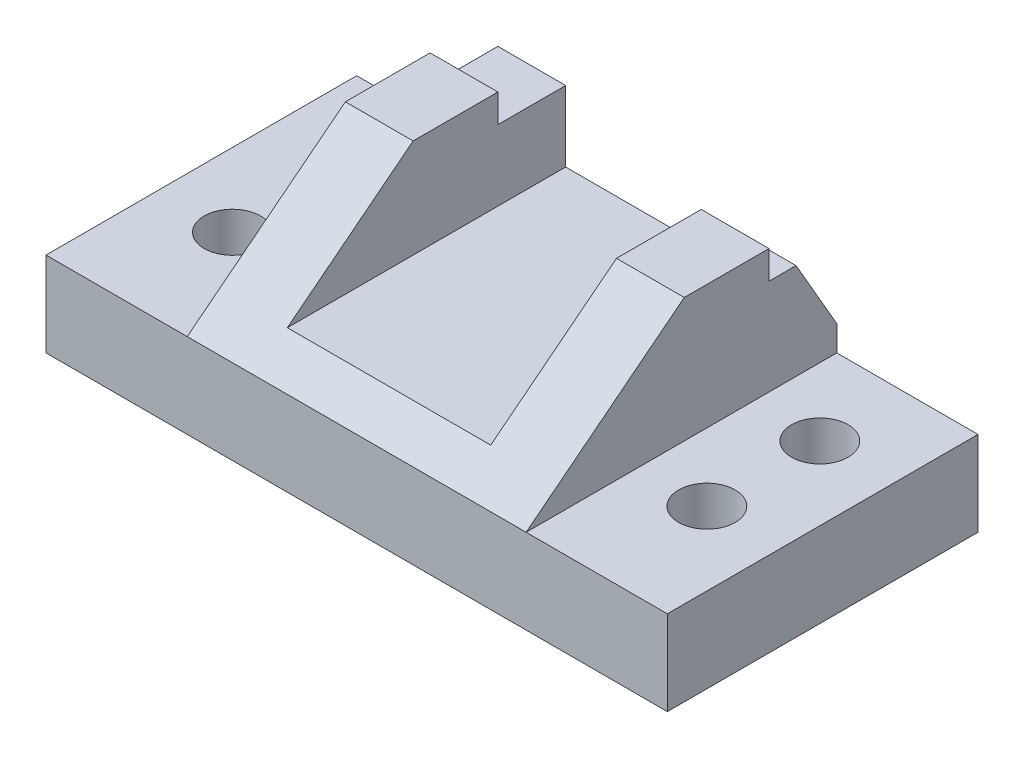
ISO-10303-21;
HEADER;
FILE_DESCRIPTION(('STEP AP214'),'2;1');
FILE_NAME('part.step','',(''),(''),'','','');
FILE_SCHEMA(('AUTOMOTIVE_DESIGN { 1 0 10303 214 1 1 1 1 }'));
ENDSEC;
DATA;
#1=APPLICATION_CONTEXT('core data for automotive mechanical design processes');
#2=APPLICATION_PROTOCOL_DEFINITION('international standard','automotive_design',2000,#1);
#3=PRODUCT_CONTEXT('',#1,'mechanical');
#4=PRODUCT('Part','Part','',(#3));
#5=PRODUCT_RELATED_PRODUCT_CATEGORY('part','',(#4));
#6=PRODUCT_DEFINITION_FORMATION('','',#4);
#7=PRODUCT_DEFINITION_CONTEXT('part definition',#1,'design');
#8=PRODUCT_DEFINITION('design','',#6,#7);
#9=PRODUCT_DEFINITION_SHAPE('','',#8);
#10=(LENGTH_UNIT() NAMED_UNIT(*) SI_UNIT(.MILLI.,.METRE.));
#11=(NAMED_UNIT(*) PLANE_ANGLE_UNIT() SI_UNIT($,.RADIAN.));
#12=(NAMED_UNIT(*) SI_UNIT($,.STERADIAN.) SOLID_ANGLE_UNIT());
#13=UNCERTAINTY_MEASURE_WITH_UNIT(LENGTH_MEASURE(1.E-05),#10,'distance_accuracy_value','');
#14=(GEOMETRIC_REPRESENTATION_CONTEXT(3) GLOBAL_UNCERTAINTY_ASSIGNED_CONTEXT((#13)) GLOBAL_UNIT_ASSIGNED_CONTEXT((#10,
#11,#12)) REPRESENTATION_CONTEXT('',''));
#15=CARTESIAN_POINT('',(0.,0.,0.));
#16=DIRECTION('',(0.,0.,1.));
#17=DIRECTION('',(1.,0.,0.));
#18=AXIS2_PLACEMENT_3D('',#15,#16,#17);
#19=CARTESIAN_POINT('',(0.,15.,0.));
#20=DIRECTION('',(0.,-1.,0.));
#21=DIRECTION('',(0.,0.,-1.));
#22=AXIS2_PLACEMENT_3D('',#19,#20,#21);
#23=PLANE('',#22);
#24=CARTESIAN_POINT('',(42.,15.,-40.));
#25=DIRECTION('',(0.,1.,0.));
#26=DIRECTION('',(0.,0.,-1.));
#27=AXIS2_PLACEMENT_3D('',#24,#25,#26);
#28=CIRCLE('',#27,5.);
#29=CARTESIAN_POINT('',(42.,15.,-45.));
#30=VERTEX_POINT('',#29);
#31=EDGE_CURVE('E229',#30,#30,#28,.T.);
#32=ORIENTED_EDGE('',*,*,#31,.F.);
#33=EDGE_LOOP('',(#32));
#34=FACE_BOUND('',#33,.T.);
#35=CARTESIAN_POINT('',(42.,15.,-20.));
#36=DIRECTION('',(0.,1.,0.));
#37=DIRECTION('',(0.,0.,-1.));
#38=AXIS2_PLACEMENT_3D('',#35,#36,#37);
#39=CIRCLE('',#38,5.);
#40=CARTESIAN_POINT('',(42.,15.,-25.));
#41=VERTEX_POINT('',#40);
#42=EDGE_CURVE('E231',#41,#41,#39,.T.);
#43=ORIENTED_EDGE('',*,*,#42,.F.);
#44=EDGE_LOOP('',(#43));
#45=FACE_BOUND('',#44,.T.);
#46=DIRECTION('',(0.,0.,-1.));
#47=VECTOR('',#46,1.);
#48=CARTESIAN_POINT('',(30.,15.,63.9061812346818));
#49=LINE('',#48,#47);
#50=CARTESIAN_POINT('',(30.,15.,0.));
#51=VERTEX_POINT('',#50);
#52=CARTESIAN_POINT('',(30.,15.,-55.));
#53=VERTEX_POINT('',#52);
#54=EDGE_CURVE('E202',#51,#53,#49,.T.);
#55=ORIENTED_EDGE('',*,*,#54,.F.);
#56=DIRECTION('',(1.,0.,0.));
#57=VECTOR('',#56,1.);
#58=CARTESIAN_POINT('',(-55.,15.,0.));
#59=LINE('',#58,#57);
#60=CARTESIAN_POINT('',(55.,15.,0.));
#61=VERTEX_POINT('',#60);
#62=EDGE_CURVE('E254',#51,#61,#59,.T.);
#63=ORIENTED_EDGE('',*,*,#62,.T.);
#64=DIRECTION('',(0.,0.,-1.));
#65=VECTOR('',#64,1.);
#66=CARTESIAN_POINT('',(55.,15.,0.));
#67=LINE('',#66,#65);
#68=CARTESIAN_POINT('',(55.,15.,-55.));
#69=VERTEX_POINT('',#68);
#70=EDGE_CURVE('E257',#61,#69,#67,.T.);
#71=ORIENTED_EDGE('',*,*,#70,.T.);
#72=DIRECTION('',(-1.,0.,0.));
#73=VECTOR('',#72,1.);
#74=CARTESIAN_POINT('',(-55.,15.,-55.));
#75=LINE('',#74,#73);
#76=EDGE_CURVE('E263',#69,#53,#75,.T.);
#77=ORIENTED_EDGE('',*,*,#76,.T.);
#78=EDGE_LOOP('',(#55,#63,#71,#77));
#79=FACE_BOUND('',#78,.T.);
#80=ADVANCED_FACE('F39',(#34,#45,#79),#23,.F.);
#81=CARTESIAN_POINT('',(-55.,15.,0.));
#82=VERTEX_POINT('',#81);
#83=CARTESIAN_POINT('',(-30.,15.,0.));
#84=VERTEX_POINT('',#83);
#85=EDGE_CURVE('E260',#82,#84,#59,.T.);
#86=ORIENTED_EDGE('',*,*,#85,.T.);
#87=DIRECTION('',(0.,0.,-1.));
#88=VECTOR('',#87,1.);
#89=CARTESIAN_POINT('',(-30.,15.,63.9061812346818));
#90=LINE('',#89,#88);
#91=CARTESIAN_POINT('',(-30.,15.,-55.));
#92=VERTEX_POINT('',#91);
#93=EDGE_CURVE('E223',#84,#92,#90,.T.);
#94=ORIENTED_EDGE('',*,*,#93,.T.);
#95=CARTESIAN_POINT('',(-55.,15.,-55.));
#96=VERTEX_POINT('',#95);
#97=EDGE_CURVE('E265',#92,#96,#75,.T.);
#98=ORIENTED_EDGE('',*,*,#97,.T.);
#99=DIRECTION('',(0.,0.,1.));
#100=VECTOR('',#99,1.);
#101=CARTESIAN_POINT('',(-55.,15.,0.));
#102=LINE('',#101,#100);
#103=EDGE_CURVE('E252',#96,#82,#102,.T.);
#104=ORIENTED_EDGE('',*,*,#103,.T.);
#105=EDGE_LOOP('',(#86,#94,#98,#104));
#106=FACE_BOUND('',#105,.T.);
#107=CARTESIAN_POINT('',(-42.,15.,-40.));
#108=DIRECTION('',(0.,1.,0.));
#109=DIRECTION('',(0.,0.,1.));
#110=AXIS2_PLACEMENT_3D('',#107,#108,#109);
#111=CIRCLE('',#110,5.);
#112=CARTESIAN_POINT('',(-42.,15.,-35.));
#113=VERTEX_POINT('',#112);
#114=EDGE_CURVE('E247',#113,#113,#111,.T.);
#115=ORIENTED_EDGE('',*,*,#114,.F.);
#116=EDGE_LOOP('',(#115));
#117=FACE_BOUND('',#116,.T.);
#118=CARTESIAN_POINT('',(-42.,15.,-20.));
#119=DIRECTION('',(0.,1.,0.));
#120=DIRECTION('',(0.,0.,1.));
#121=AXIS2_PLACEMENT_3D('',#118,#119,#120);
#122=CIRCLE('',#121,5.);
#123=CARTESIAN_POINT('',(-42.,15.,-15.));
#124=VERTEX_POINT('',#123);
#125=EDGE_CURVE('E238',#124,#124,#122,.T.);
#126=ORIENTED_EDGE('',*,*,#125,.F.);
#127=EDGE_LOOP('',(#126));
#128=FACE_BOUND('',#127,.T.);
#129=ADVANCED_FACE('F302',(#106,#117,#128),#23,.F.);
#130=CARTESIAN_POINT('',(0.,0.,0.));
#131=DIRECTION('',(0.,-1.,0.));
#132=DIRECTION('',(0.,0.,-1.));
#133=AXIS2_PLACEMENT_3D('',#130,#131,#132);
#134=PLANE('',#133);
#135=CARTESIAN_POINT('',(42.,0.,-20.));
#136=DIRECTION('',(0.,1.,0.));
#137=DIRECTION('',(0.,0.,-1.));
#138=AXIS2_PLACEMENT_3D('',#135,#136,#137);
#139=CIRCLE('',#138,5.);
#140=CARTESIAN_POINT('',(42.,0.,-25.));
#141=VERTEX_POINT('',#140);
#142=EDGE_CURVE('E232',#141,#141,#139,.T.);
#143=ORIENTED_EDGE('',*,*,#142,.T.);
#144=EDGE_LOOP('',(#143));
#145=FACE_BOUND('',#144,.T.);
#146=CARTESIAN_POINT('',(-42.,0.,-40.));
#147=DIRECTION('',(0.,1.,0.));
#148=DIRECTION('',(0.,0.,1.));
#149=AXIS2_PLACEMENT_3D('',#146,#147,#148);
#150=CIRCLE('',#149,5.);
#151=CARTESIAN_POINT('',(-42.,0.,-35.));
#152=VERTEX_POINT('',#151);
#153=EDGE_CURVE('E244',#152,#152,#150,.T.);
#154=ORIENTED_EDGE('',*,*,#153,.T.);
#155=EDGE_LOOP('',(#154));
#156=FACE_BOUND('',#155,.T.);
#157=DIRECTION('',(0.,0.,1.));
#158=VECTOR('',#157,1.);
#159=CARTESIAN_POINT('',(-55.,0.,0.));
#160=LINE('',#159,#158);
#161=CARTESIAN_POINT('',(-55.,0.,-55.));
#162=VERTEX_POINT('',#161);
#163=CARTESIAN_POINT('',(-55.,0.,0.));
#164=VERTEX_POINT('',#163);
#165=EDGE_CURVE('E246',#162,#164,#160,.T.);
#166=ORIENTED_EDGE('',*,*,#165,.F.);
#167=DIRECTION('',(-1.,0.,0.));
#168=VECTOR('',#167,1.);
#169=CARTESIAN_POINT('',(-55.,0.,-55.));
#170=LINE('',#169,#168);
#171=CARTESIAN_POINT('',(55.,0.,-55.));
#172=VERTEX_POINT('',#171);
#173=EDGE_CURVE('E258',#172,#162,#170,.T.);
#174=ORIENTED_EDGE('',*,*,#173,.F.);
#175=DIRECTION('',(0.,0.,-1.));
#176=VECTOR('',#175,1.);
#177=CARTESIAN_POINT('',(55.,0.,0.));
#178=LINE('',#177,#176);
#179=CARTESIAN_POINT('',(55.,0.,0.));
#180=VERTEX_POINT('',#179);
#181=EDGE_CURVE('E271',#180,#172,#178,.T.);
#182=ORIENTED_EDGE('',*,*,#181,.F.);
#183=DIRECTION('',(1.,0.,0.));
#184=VECTOR('',#183,1.);
#185=CARTESIAN_POINT('',(-55.,0.,0.));
#186=LINE('',#185,#184);
#187=EDGE_CURVE('E267',#164,#180,#186,.T.);
#188=ORIENTED_EDGE('',*,*,#187,.F.);
#189=EDGE_LOOP('',(#166,#174,#182,#188));
#190=FACE_BOUND('',#189,.T.);
#191=CARTESIAN_POINT('',(-42.,0.,-20.));
#192=DIRECTION('',(0.,1.,0.));
#193=DIRECTION('',(0.,0.,1.));
#194=AXIS2_PLACEMENT_3D('',#191,#192,#193);
#195=CIRCLE('',#194,5.);
#196=CARTESIAN_POINT('',(-42.,0.,-15.));
#197=VERTEX_POINT('',#196);
#198=EDGE_CURVE('E240',#197,#197,#195,.T.);
#199=ORIENTED_EDGE('',*,*,#198,.T.);
#200=EDGE_LOOP('',(#199));
#201=FACE_BOUND('',#200,.T.);
#202=CARTESIAN_POINT('',(42.,0.,-40.));
#203=DIRECTION('',(0.,1.,0.));
#204=DIRECTION('',(0.,0.,-1.));
#205=AXIS2_PLACEMENT_3D('',#202,#203,#204);
#206=CIRCLE('',#205,5.);
#207=CARTESIAN_POINT('',(42.,0.,-45.));
#208=VERTEX_POINT('',#207);
#209=EDGE_CURVE('E207',#208,#208,#206,.T.);
#210=ORIENTED_EDGE('',*,*,#209,.T.);
#211=EDGE_LOOP('',(#210));
#212=FACE_BOUND('',#211,.T.);
#213=ADVANCED_FACE('F288',(#145,#156,#190,#201,#212),#134,.T.);
#214=CARTESIAN_POINT('',(-55.,15.,0.));
#215=DIRECTION('',(1.,0.,0.));
#216=DIRECTION('',(0.,0.,-1.));
#217=AXIS2_PLACEMENT_3D('',#214,#215,#216);
#218=PLANE('',#217);
#219=ORIENTED_EDGE('',*,*,#165,.T.);
#220=DIRECTION('',(0.,-1.,0.));
#221=VECTOR('',#220,1.);
#222=CARTESIAN_POINT('',(-55.,15.,0.));
#223=LINE('',#222,#221);
#224=EDGE_CURVE('E11',#82,#164,#223,.T.);
#225=ORIENTED_EDGE('',*,*,#224,.F.);
#226=ORIENTED_EDGE('',*,*,#103,.F.);
#227=DIRECTION('',(0.,-1.,0.));
#228=VECTOR('',#227,1.);
#229=CARTESIAN_POINT('',(-55.,15.,-55.));
#230=LINE('',#229,#228);
#231=EDGE_CURVE('E266',#96,#162,#230,.T.);
#232=ORIENTED_EDGE('',*,*,#231,.T.);
#233=EDGE_LOOP('',(#219,#225,#226,#232));
#234=FACE_BOUND('',#233,.T.);
#235=ADVANCED_FACE('F41',(#234),#218,.F.);
#236=CARTESIAN_POINT('',(-55.,15.,0.));
#237=DIRECTION('',(0.,0.,-1.));
#238=DIRECTION('',(-1.,0.,0.));
#239=AXIS2_PLACEMENT_3D('',#236,#237,#238);
#240=PLANE('',#239);
#241=ORIENTED_EDGE('',*,*,#62,.F.);
#242=DIRECTION('',(-1.,0.,0.));
#243=VECTOR('',#242,1.);
#244=CARTESIAN_POINT('',(55.,15.,0.));
#245=LINE('',#244,#243);
#246=EDGE_CURVE('E318',#51,#84,#245,.T.);
#247=ORIENTED_EDGE('',*,*,#246,.T.);
#248=ORIENTED_EDGE('',*,*,#85,.F.);
#249=ORIENTED_EDGE('',*,*,#224,.T.);
#250=ORIENTED_EDGE('',*,*,#187,.T.);
#251=DIRECTION('',(0.,-1.,0.));
#252=VECTOR('',#251,1.);
#253=CARTESIAN_POINT('',(55.,15.,0.));
#254=LINE('',#253,#252);
#255=EDGE_CURVE('E50',#61,#180,#254,.T.);
#256=ORIENTED_EDGE('',*,*,#255,.F.);
#257=EDGE_LOOP('',(#241,#247,#248,#249,#250,#256));
#258=FACE_BOUND('',#257,.T.);
#259=ADVANCED_FACE('F358',(#258),#240,.F.);
#260=CARTESIAN_POINT('',(55.,15.,0.));
#261=DIRECTION('',(-1.,0.,0.));
#262=DIRECTION('',(0.,0.,1.));
#263=AXIS2_PLACEMENT_3D('',#260,#261,#262);
#264=PLANE('',#263);
#265=ORIENTED_EDGE('',*,*,#181,.T.);
#266=DIRECTION('',(0.,-1.,0.));
#267=VECTOR('',#266,1.);
#268=CARTESIAN_POINT('',(55.,15.,-55.));
#269=LINE('',#268,#267);
#270=EDGE_CURVE('E277',#69,#172,#269,.T.);
#271=ORIENTED_EDGE('',*,*,#270,.F.);
#272=ORIENTED_EDGE('',*,*,#70,.F.);
#273=ORIENTED_EDGE('',*,*,#255,.T.);
#274=EDGE_LOOP('',(#265,#271,#272,#273));
#275=FACE_BOUND('',#274,.T.);
#276=ADVANCED_FACE('F284',(#275),#264,.F.);
#277=CARTESIAN_POINT('',(-55.,15.,-55.));
#278=DIRECTION('',(0.,0.,1.));
#279=DIRECTION('',(1.,0.,0.));
#280=AXIS2_PLACEMENT_3D('',#277,#278,#279);
#281=PLANE('',#280);
#282=DIRECTION('',(1.,0.,0.));
#283=VECTOR('',#282,1.);
#284=CARTESIAN_POINT('',(-18.,19.5,-55.));
#285=LINE('',#284,#283);
#286=CARTESIAN_POINT('',(-18.,19.5,-55.));
#287=VERTEX_POINT('',#286);
#288=CARTESIAN_POINT('',(18.,19.5,-55.));
#289=VERTEX_POINT('',#288);
#290=EDGE_CURVE('E205',#287,#289,#285,.T.);
#291=ORIENTED_EDGE('',*,*,#290,.T.);
#292=DIRECTION('',(-1.,0.,0.));
#293=VECTOR('',#292,1.);
#294=CARTESIAN_POINT('',(44.4337567297406,19.5,-55.));
#295=LINE('',#294,#293);
#296=CARTESIAN_POINT('',(30.,19.5,-55.));
#297=VERTEX_POINT('',#296);
#298=EDGE_CURVE('E161',#297,#289,#295,.T.);
#299=ORIENTED_EDGE('',*,*,#298,.F.);
#300=DIRECTION('',(0.,-1.,0.));
#301=VECTOR('',#300,1.);
#302=CARTESIAN_POINT('',(30.,15.,-55.));
#303=LINE('',#302,#301);
#304=EDGE_CURVE('E168',#297,#53,#303,.T.);
#305=ORIENTED_EDGE('',*,*,#304,.T.);
#306=ORIENTED_EDGE('',*,*,#76,.F.);
#307=ORIENTED_EDGE('',*,*,#270,.T.);
#308=ORIENTED_EDGE('',*,*,#173,.T.);
#309=ORIENTED_EDGE('',*,*,#231,.F.);
#310=ORIENTED_EDGE('',*,*,#97,.F.);
#311=DIRECTION('',(0.,1.,0.));
#312=VECTOR('',#311,1.);
#313=CARTESIAN_POINT('',(-30.,15.,-55.));
#314=LINE('',#313,#312);
#315=CARTESIAN_POINT('',(-30.,32.,-55.));
#316=VERTEX_POINT('',#315);
#317=EDGE_CURVE('E197',#92,#316,#314,.T.);
#318=ORIENTED_EDGE('',*,*,#317,.T.);
#319=DIRECTION('',(-1.,0.,0.));
#320=VECTOR('',#319,1.);
#321=CARTESIAN_POINT('',(55.,32.,-55.));
#322=LINE('',#321,#320);
#323=CARTESIAN_POINT('',(-18.,32.,-55.));
#324=VERTEX_POINT('',#323);
#325=EDGE_CURVE('E62',#324,#316,#322,.T.);
#326=ORIENTED_EDGE('',*,*,#325,.F.);
#327=DIRECTION('',(0.,-1.,0.));
#328=VECTOR('',#327,1.);
#329=CARTESIAN_POINT('',(-18.,19.5,-55.));
#330=LINE('',#329,#328);
#331=EDGE_CURVE('E199',#324,#287,#330,.T.);
#332=ORIENTED_EDGE('',*,*,#331,.T.);
#333=EDGE_LOOP('',(#291,#299,#305,#306,#307,#308,#309,#310,#318,#326,#332));
#334=FACE_BOUND('',#333,.T.);
#335=ADVANCED_FACE('F294',(#334),#281,.F.);
#336=CARTESIAN_POINT('',(-42.,15.,-40.));
#337=DIRECTION('',(0.,-1.,0.));
#338=DIRECTION('',(0.,0.,-1.));
#339=AXIS2_PLACEMENT_3D('',#336,#337,#338);
#340=CYLINDRICAL_SURFACE('',#339,5.);
#341=ORIENTED_EDGE('',*,*,#114,.T.);
#342=EDGE_LOOP('',(#341));
#343=FACE_BOUND('',#342,.T.);
#344=ORIENTED_EDGE('',*,*,#153,.F.);
#345=EDGE_LOOP('',(#344));
#346=FACE_BOUND('',#345,.T.);
#347=ADVANCED_FACE('F377',(#343,#346),#340,.F.);
#348=CARTESIAN_POINT('',(-42.,15.,-20.));
#349=DIRECTION('',(0.,-1.,0.));
#350=DIRECTION('',(0.,0.,-1.));
#351=AXIS2_PLACEMENT_3D('',#348,#349,#350);
#352=CYLINDRICAL_SURFACE('',#351,5.);
#353=ORIENTED_EDGE('',*,*,#125,.T.);
#354=EDGE_LOOP('',(#353));
#355=FACE_BOUND('',#354,.T.);
#356=ORIENTED_EDGE('',*,*,#198,.F.);
#357=EDGE_LOOP('',(#356));
#358=FACE_BOUND('',#357,.T.);
#359=ADVANCED_FACE('F388',(#355,#358),#352,.F.);
#360=CARTESIAN_POINT('',(42.,15.,-20.));
#361=DIRECTION('',(0.,-1.,0.));
#362=DIRECTION('',(0.,0.,-1.));
#363=AXIS2_PLACEMENT_3D('',#360,#361,#362);
#364=CYLINDRICAL_SURFACE('',#363,5.);
#365=ORIENTED_EDGE('',*,*,#42,.T.);
#366=EDGE_LOOP('',(#365));
#367=FACE_BOUND('',#366,.T.);
#368=ORIENTED_EDGE('',*,*,#142,.F.);
#369=EDGE_LOOP('',(#368));
#370=FACE_BOUND('',#369,.T.);
#371=ADVANCED_FACE('F395',(#367,#370),#364,.F.);
#372=CARTESIAN_POINT('',(42.,15.,-40.));
#373=DIRECTION('',(0.,-1.,0.));
#374=DIRECTION('',(0.,0.,-1.));
#375=AXIS2_PLACEMENT_3D('',#372,#373,#374);
#376=CYLINDRICAL_SURFACE('',#375,5.);
#377=ORIENTED_EDGE('',*,*,#31,.T.);
#378=EDGE_LOOP('',(#377));
#379=FACE_BOUND('',#378,.T.);
#380=ORIENTED_EDGE('',*,*,#209,.F.);
#381=EDGE_LOOP('',(#380));
#382=FACE_BOUND('',#381,.T.);
#383=ADVANCED_FACE('F409',(#379,#382),#376,.F.);
#384=CARTESIAN_POINT('',(30.,15.,63.9061812346818));
#385=DIRECTION('',(1.,0.,0.));
#386=DIRECTION('',(0.,0.,-1.));
#387=AXIS2_PLACEMENT_3D('',#384,#385,#386);
#388=PLANE('',#387);
#389=DIRECTION('',(0.,0.866025403784442,0.499999999999995));
#390=VECTOR('',#389,1.);
#391=CARTESIAN_POINT('',(30.,19.5,-55.));
#392=LINE('',#391,#390);
#393=CARTESIAN_POINT('',(30.,32.,-47.7831216351298));
#394=VERTEX_POINT('',#393);
#395=EDGE_CURVE('E156',#297,#394,#392,.T.);
#396=ORIENTED_EDGE('',*,*,#395,.T.);
#397=DIRECTION('',(0.,0.,-1.));
#398=VECTOR('',#397,1.);
#399=CARTESIAN_POINT('',(30.,32.,63.9061812346818));
#400=LINE('',#399,#398);
#401=CARTESIAN_POINT('',(30.,32.,-43.));
#402=VERTEX_POINT('',#401);
#403=EDGE_CURVE('E169',#402,#394,#400,.T.);
#404=ORIENTED_EDGE('',*,*,#403,.F.);
#405=DIRECTION('',(0.,-1.,0.));
#406=VECTOR('',#405,1.);
#407=CARTESIAN_POINT('',(30.,15.,-43.));
#408=LINE('',#407,#406);
#409=CARTESIAN_POINT('',(30.,37.,-43.));
#410=VERTEX_POINT('',#409);
#411=EDGE_CURVE('E186',#410,#402,#408,.T.);
#412=ORIENTED_EDGE('',*,*,#411,.F.);
#413=DIRECTION('',(0.,0.,-1.));
#414=VECTOR('',#413,1.);
#415=CARTESIAN_POINT('',(30.,37.,63.9061812346818));
#416=LINE('',#415,#414);
#417=CARTESIAN_POINT('',(30.,37.,-28.));
#418=VERTEX_POINT('',#417);
#419=EDGE_CURVE('E206',#418,#410,#416,.T.);
#420=ORIENTED_EDGE('',*,*,#419,.F.);
#421=DIRECTION('',(0.,0.617821551931904,-0.786318338822423));
#422=VECTOR('',#421,1.);
#423=CARTESIAN_POINT('',(30.,-16.0459050793092,39.5129701009389));
#424=LINE('',#423,#422);
#425=EDGE_CURVE('E191',#51,#418,#424,.T.);
#426=ORIENTED_EDGE('',*,*,#425,.F.);
#427=ORIENTED_EDGE('',*,*,#54,.T.);
#428=ORIENTED_EDGE('',*,*,#304,.F.);
#429=EDGE_LOOP('',(#396,#404,#412,#420,#426,#427,#428));
#430=FACE_BOUND('',#429,.T.);
#431=ADVANCED_FACE('F167',(#430),#388,.T.);
#432=CARTESIAN_POINT('',(30.,37.,63.9061812346818));
#433=DIRECTION('',(0.,1.,0.));
#434=DIRECTION('',(0.,0.,1.));
#435=AXIS2_PLACEMENT_3D('',#432,#433,#434);
#436=PLANE('',#435);
#437=DIRECTION('',(-1.,0.,0.));
#438=VECTOR('',#437,1.);
#439=CARTESIAN_POINT('',(55.,37.,-28.));
#440=LINE('',#439,#438);
#441=CARTESIAN_POINT('',(18.,37.,-28.));
#442=VERTEX_POINT('',#441);
#443=EDGE_CURVE('E321',#418,#442,#440,.T.);
#444=ORIENTED_EDGE('',*,*,#443,.F.);
#445=ORIENTED_EDGE('',*,*,#419,.T.);
#446=DIRECTION('',(-1.,0.,0.));
#447=VECTOR('',#446,1.);
#448=CARTESIAN_POINT('',(55.,37.,-43.));
#449=LINE('',#448,#447);
#450=CARTESIAN_POINT('',(18.,37.,-43.));
#451=VERTEX_POINT('',#450);
#452=EDGE_CURVE('E327',#410,#451,#449,.T.);
#453=ORIENTED_EDGE('',*,*,#452,.T.);
#454=DIRECTION('',(0.,0.,-1.));
#455=VECTOR('',#454,1.);
#456=CARTESIAN_POINT('',(18.,37.,63.9061812346818));
#457=LINE('',#456,#455);
#458=EDGE_CURVE('E209',#442,#451,#457,.T.);
#459=ORIENTED_EDGE('',*,*,#458,.F.);
#460=EDGE_LOOP('',(#444,#445,#453,#459));
#461=FACE_BOUND('',#460,.T.);
#462=ADVANCED_FACE('F411',(#461),#436,.T.);
#463=CARTESIAN_POINT('',(18.,19.5,63.9061812346818));
#464=DIRECTION('',(-1.,0.,0.));
#465=DIRECTION('',(0.,0.,1.));
#466=AXIS2_PLACEMENT_3D('',#463,#464,#465);
#467=PLANE('',#466);
#468=DIRECTION('',(0.,0.866025403784442,0.499999999999995));
#469=VECTOR('',#468,1.);
#470=CARTESIAN_POINT('',(18.,19.5,-55.));
#471=LINE('',#470,#469);
#472=CARTESIAN_POINT('',(18.,32.,-47.7831216351298));
#473=VERTEX_POINT('',#472);
#474=EDGE_CURVE('E53',#289,#473,#471,.T.);
#475=ORIENTED_EDGE('',*,*,#474,.F.);
#476=DIRECTION('',(0.,0.,-1.));
#477=VECTOR('',#476,1.);
#478=CARTESIAN_POINT('',(18.,19.5,63.9061812346818));
#479=LINE('',#478,#477);
#480=CARTESIAN_POINT('',(18.,19.5,-5.72727272727275));
#481=VERTEX_POINT('',#480);
#482=EDGE_CURVE('E213',#481,#289,#479,.T.);
#483=ORIENTED_EDGE('',*,*,#482,.F.);
#484=DIRECTION('',(0.,-0.617821551931904,0.786318338822423));
#485=VECTOR('',#484,1.);
#486=CARTESIAN_POINT('',(18.,-14.3282394641672,37.3268502271219));
#487=LINE('',#486,#485);
#488=EDGE_CURVE('E194',#442,#481,#487,.T.);
#489=ORIENTED_EDGE('',*,*,#488,.F.);
#490=ORIENTED_EDGE('',*,*,#458,.T.);
#491=DIRECTION('',(0.,1.,0.));
#492=VECTOR('',#491,1.);
#493=CARTESIAN_POINT('',(18.,19.5,-43.));
#494=LINE('',#493,#492);
#495=CARTESIAN_POINT('',(18.,32.,-43.));
#496=VERTEX_POINT('',#495);
#497=EDGE_CURVE('E176',#496,#451,#494,.T.);
#498=ORIENTED_EDGE('',*,*,#497,.F.);
#499=DIRECTION('',(0.,0.,1.));
#500=VECTOR('',#499,1.);
#501=CARTESIAN_POINT('',(18.,32.,63.9061812346818));
#502=LINE('',#501,#500);
#503=EDGE_CURVE('E179',#473,#496,#502,.T.);
#504=ORIENTED_EDGE('',*,*,#503,.F.);
#505=EDGE_LOOP('',(#475,#483,#489,#490,#498,#504));
#506=FACE_BOUND('',#505,.T.);
#507=ADVANCED_FACE('F337',(#506),#467,.T.);
#508=CARTESIAN_POINT('',(-18.,19.5,63.9061812346818));
#509=DIRECTION('',(0.,1.,0.));
#510=DIRECTION('',(0.,0.,1.));
#511=AXIS2_PLACEMENT_3D('',#508,#509,#510);
#512=PLANE('',#511);
#513=DIRECTION('',(-1.,0.,0.));
#514=VECTOR('',#513,1.);
#515=CARTESIAN_POINT('',(-18.,19.5,-5.72727272727275));
#516=LINE('',#515,#514);
#517=CARTESIAN_POINT('',(-18.,19.5,-5.72727272727277));
#518=VERTEX_POINT('',#517);
#519=EDGE_CURVE('E190',#481,#518,#516,.T.);
#520=ORIENTED_EDGE('',*,*,#519,.F.);
#521=ORIENTED_EDGE('',*,*,#482,.T.);
#522=ORIENTED_EDGE('',*,*,#290,.F.);
#523=DIRECTION('',(0.,0.,-1.));
#524=VECTOR('',#523,1.);
#525=CARTESIAN_POINT('',(-18.,19.5,63.9061812346818));
#526=LINE('',#525,#524);
#527=EDGE_CURVE('E216',#518,#287,#526,.T.);
#528=ORIENTED_EDGE('',*,*,#527,.F.);
#529=EDGE_LOOP('',(#520,#521,#522,#528));
#530=FACE_BOUND('',#529,.T.);
#531=ADVANCED_FACE('F345',(#530),#512,.T.);
#532=CARTESIAN_POINT('',(-18.,19.5,63.9061812346818));
#533=DIRECTION('',(1.,0.,0.));
#534=DIRECTION('',(0.,1.,0.));
#535=AXIS2_PLACEMENT_3D('',#532,#533,#534);
#536=PLANE('',#535);
#537=DIRECTION('',(0.,0.617821551931904,-0.786318338822423));
#538=VECTOR('',#537,1.);
#539=CARTESIAN_POINT('',(-18.,-14.3282394641672,37.3268502271219));
#540=LINE('',#539,#538);
#541=CARTESIAN_POINT('',(-18.,37.,-28.));
#542=VERTEX_POINT('',#541);
#543=EDGE_CURVE('E189',#518,#542,#540,.T.);
#544=ORIENTED_EDGE('',*,*,#543,.F.);
#545=ORIENTED_EDGE('',*,*,#527,.T.);
#546=ORIENTED_EDGE('',*,*,#331,.F.);
#547=DIRECTION('',(0.,0.,-1.));
#548=VECTOR('',#547,1.);
#549=CARTESIAN_POINT('',(-18.,32.,63.9061812346818));
#550=LINE('',#549,#548);
#551=CARTESIAN_POINT('',(-18.,32.,-43.));
#552=VERTEX_POINT('',#551);
#553=EDGE_CURVE('E182',#552,#324,#550,.T.);
#554=ORIENTED_EDGE('',*,*,#553,.F.);
#555=DIRECTION('',(0.,-1.,0.));
#556=VECTOR('',#555,1.);
#557=CARTESIAN_POINT('',(-18.,19.5,-43.));
#558=LINE('',#557,#556);
#559=CARTESIAN_POINT('',(-18.,37.,-43.));
#560=VERTEX_POINT('',#559);
#561=EDGE_CURVE('E177',#560,#552,#558,.T.);
#562=ORIENTED_EDGE('',*,*,#561,.F.);
#563=DIRECTION('',(0.,0.,-1.));
#564=VECTOR('',#563,1.);
#565=CARTESIAN_POINT('',(-18.,37.,63.9061812346818));
#566=LINE('',#565,#564);
#567=EDGE_CURVE('E218',#542,#560,#566,.T.);
#568=ORIENTED_EDGE('',*,*,#567,.F.);
#569=EDGE_LOOP('',(#544,#545,#546,#554,#562,#568));
#570=FACE_BOUND('',#569,.T.);
#571=ADVANCED_FACE('F346',(#570),#536,.T.);
#572=CARTESIAN_POINT('',(-18.,37.,63.9061812346818));
#573=DIRECTION('',(0.,1.,0.));
#574=DIRECTION('',(-1.,0.,0.));
#575=AXIS2_PLACEMENT_3D('',#572,#573,#574);
#576=PLANE('',#575);
#577=CARTESIAN_POINT('',(-30.,37.,-28.));
#578=VERTEX_POINT('',#577);
#579=EDGE_CURVE('E314',#542,#578,#440,.T.);
#580=ORIENTED_EDGE('',*,*,#579,.F.);
#581=ORIENTED_EDGE('',*,*,#567,.T.);
#582=CARTESIAN_POINT('',(-30.,37.,-43.));
#583=VERTEX_POINT('',#582);
#584=EDGE_CURVE('E328',#560,#583,#449,.T.);
#585=ORIENTED_EDGE('',*,*,#584,.T.);
#586=DIRECTION('',(0.,0.,-1.));
#587=VECTOR('',#586,1.);
#588=CARTESIAN_POINT('',(-30.,37.,63.9061812346818));
#589=LINE('',#588,#587);
#590=EDGE_CURVE('E225',#578,#583,#589,.T.);
#591=ORIENTED_EDGE('',*,*,#590,.F.);
#592=EDGE_LOOP('',(#580,#581,#585,#591));
#593=FACE_BOUND('',#592,.T.);
#594=ADVANCED_FACE('F353',(#593),#576,.T.);
#595=CARTESIAN_POINT('',(-30.,15.,63.9061812346818));
#596=DIRECTION('',(-1.,0.,0.));
#597=DIRECTION('',(0.,0.,1.));
#598=AXIS2_PLACEMENT_3D('',#595,#596,#597);
#599=PLANE('',#598);
#600=DIRECTION('',(0.,-0.617821551931904,0.786318338822423));
#601=VECTOR('',#600,1.);
#602=CARTESIAN_POINT('',(-30.,15.,0.));
#603=LINE('',#602,#601);
#604=EDGE_CURVE('E315',#578,#84,#603,.T.);
#605=ORIENTED_EDGE('',*,*,#604,.F.);
#606=ORIENTED_EDGE('',*,*,#590,.T.);
#607=DIRECTION('',(0.,1.,0.));
#608=VECTOR('',#607,1.);
#609=CARTESIAN_POINT('',(-30.,37.,-43.));
#610=LINE('',#609,#608);
#611=CARTESIAN_POINT('',(-30.,32.,-43.));
#612=VERTEX_POINT('',#611);
#613=EDGE_CURVE('E309',#612,#583,#610,.T.);
#614=ORIENTED_EDGE('',*,*,#613,.F.);
#615=DIRECTION('',(0.,0.,1.));
#616=VECTOR('',#615,1.);
#617=CARTESIAN_POINT('',(-30.,32.,-43.));
#618=LINE('',#617,#616);
#619=EDGE_CURVE('E310',#316,#612,#618,.T.);
#620=ORIENTED_EDGE('',*,*,#619,.F.);
#621=ORIENTED_EDGE('',*,*,#317,.F.);
#622=ORIENTED_EDGE('',*,*,#93,.F.);
#623=EDGE_LOOP('',(#605,#606,#614,#620,#621,#622));
#624=FACE_BOUND('',#623,.T.);
#625=ADVANCED_FACE('F307',(#624),#599,.T.);
#626=CARTESIAN_POINT('',(55.,32.,-43.));
#627=DIRECTION('',(0.,-1.,0.));
#628=DIRECTION('',(0.,0.,-1.));
#629=AXIS2_PLACEMENT_3D('',#626,#627,#628);
#630=PLANE('',#629);
#631=ORIENTED_EDGE('',*,*,#553,.T.);
#632=ORIENTED_EDGE('',*,*,#325,.T.);
#633=ORIENTED_EDGE('',*,*,#619,.T.);
#634=DIRECTION('',(-1.,0.,0.));
#635=VECTOR('',#634,1.);
#636=CARTESIAN_POINT('',(55.,32.,-43.));
#637=LINE('',#636,#635);
#638=EDGE_CURVE('E330',#552,#612,#637,.T.);
#639=ORIENTED_EDGE('',*,*,#638,.F.);
#640=EDGE_LOOP('',(#631,#632,#633,#639));
#641=FACE_BOUND('',#640,.T.);
#642=ADVANCED_FACE('F423',(#641),#630,.F.);
#643=CARTESIAN_POINT('',(55.,37.,-43.));
#644=DIRECTION('',(0.,0.,1.));
#645=DIRECTION('',(1.,0.,0.));
#646=AXIS2_PLACEMENT_3D('',#643,#644,#645);
#647=PLANE('',#646);
#648=ORIENTED_EDGE('',*,*,#561,.T.);
#649=ORIENTED_EDGE('',*,*,#638,.T.);
#650=ORIENTED_EDGE('',*,*,#613,.T.);
#651=ORIENTED_EDGE('',*,*,#584,.F.);
#652=EDGE_LOOP('',(#648,#649,#650,#651));
#653=FACE_BOUND('',#652,.T.);
#654=ADVANCED_FACE('F435',(#653),#647,.F.);
#655=CARTESIAN_POINT('',(55.,15.,0.));
#656=DIRECTION('',(0.,-0.786318338822423,-0.617821551931904));
#657=DIRECTION('',(0.,0.617821551931904,-0.786318338822423));
#658=AXIS2_PLACEMENT_3D('',#655,#656,#657);
#659=PLANE('',#658);
#660=ORIENTED_EDGE('',*,*,#425,.T.);
#661=ORIENTED_EDGE('',*,*,#443,.T.);
#662=ORIENTED_EDGE('',*,*,#488,.T.);
#663=ORIENTED_EDGE('',*,*,#519,.T.);
#664=ORIENTED_EDGE('',*,*,#543,.T.);
#665=ORIENTED_EDGE('',*,*,#579,.T.);
#666=ORIENTED_EDGE('',*,*,#604,.T.);
#667=ORIENTED_EDGE('',*,*,#246,.F.);
#668=EDGE_LOOP('',(#660,#661,#662,#663,#664,#665,#666,#667));
#669=FACE_BOUND('',#668,.T.);
#670=ADVANCED_FACE('F354',(#669),#659,.F.);
#671=ORIENTED_EDGE('',*,*,#411,.T.);
#672=EDGE_CURVE('E175',#402,#496,#637,.T.);
#673=ORIENTED_EDGE('',*,*,#672,.T.);
#674=ORIENTED_EDGE('',*,*,#497,.T.);
#675=ORIENTED_EDGE('',*,*,#452,.F.);
#676=EDGE_LOOP('',(#671,#673,#674,#675));
#677=FACE_BOUND('',#676,.T.);
#678=ADVANCED_FACE('F436',(#677),#647,.F.);
#679=ORIENTED_EDGE('',*,*,#403,.T.);
#680=DIRECTION('',(-1.,0.,0.));
#681=VECTOR('',#680,1.);
#682=CARTESIAN_POINT('',(44.4337567297406,32.,-47.7831216351298));
#683=LINE('',#682,#681);
#684=EDGE_CURVE('E153',#394,#473,#683,.T.);
#685=ORIENTED_EDGE('',*,*,#684,.T.);
#686=ORIENTED_EDGE('',*,*,#503,.T.);
#687=ORIENTED_EDGE('',*,*,#672,.F.);
#688=EDGE_LOOP('',(#679,#685,#686,#687));
#689=FACE_BOUND('',#688,.T.);
#690=ADVANCED_FACE('F174',(#689),#630,.F.);
#691=CARTESIAN_POINT('',(44.4337567297406,19.5,-55.));
#692=DIRECTION('',(0.,-0.499999999999995,0.866025403784442));
#693=DIRECTION('',(0.,-0.866025403784442,-0.499999999999995));
#694=AXIS2_PLACEMENT_3D('',#691,#692,#693);
#695=PLANE('',#694);
#696=ORIENTED_EDGE('',*,*,#298,.T.);
#697=ORIENTED_EDGE('',*,*,#474,.T.);
#698=ORIENTED_EDGE('',*,*,#684,.F.);
#699=ORIENTED_EDGE('',*,*,#395,.F.);
#700=EDGE_LOOP('',(#696,#697,#698,#699));
#701=FACE_BOUND('',#700,.T.);
#702=ADVANCED_FACE('F154',(#701),#695,.F.);
#703=CLOSED_SHELL('',(#80,#129,#213,#235,#259,#276,#335,#347,#359,#371,#383,#431,#462,#507,#531,
#571,#594,#625,#642,#654,#670,#678,#690,#702));
#704=MANIFOLD_SOLID_BREP('B2',#703);
#705=ADVANCED_BREP_SHAPE_REPRESENTATION('',(#18,#704),#14);
#706=SHAPE_DEFINITION_REPRESENTATION(#9,#705);
ENDSEC;
END-ISO-10303-21;
